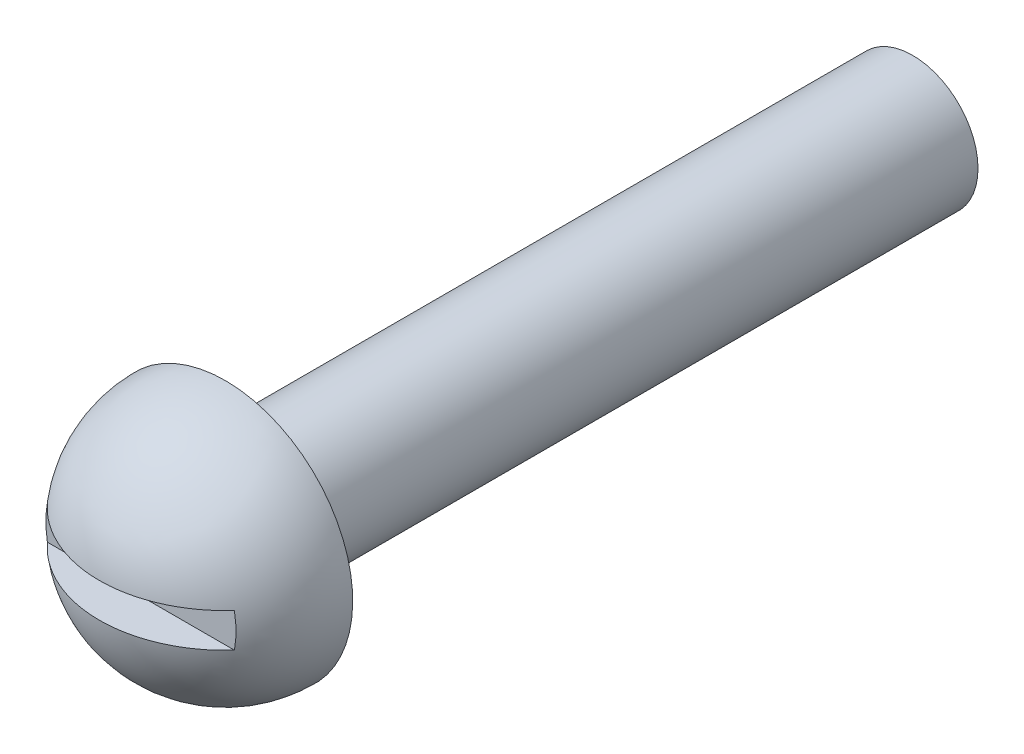
ISO-10303-21;
HEADER;
FILE_DESCRIPTION(('STEP AP214'),'2;1');
FILE_NAME('part.step','',(''),(''),'','','');
FILE_SCHEMA(('AUTOMOTIVE_DESIGN { 1 0 10303 214 1 1 1 1 }'));
ENDSEC;
DATA;
#1=APPLICATION_CONTEXT('core data for automotive mechanical design processes');
#2=APPLICATION_PROTOCOL_DEFINITION('international standard','automotive_design',2000,#1);
#3=PRODUCT_CONTEXT('',#1,'mechanical');
#4=PRODUCT('Part','Part','',(#3));
#5=PRODUCT_RELATED_PRODUCT_CATEGORY('part','',(#4));
#6=PRODUCT_DEFINITION_FORMATION('','',#4);
#7=PRODUCT_DEFINITION_CONTEXT('part definition',#1,'design');
#8=PRODUCT_DEFINITION('design','',#6,#7);
#9=PRODUCT_DEFINITION_SHAPE('','',#8);
#10=(LENGTH_UNIT() NAMED_UNIT(*) SI_UNIT(.MILLI.,.METRE.));
#11=(NAMED_UNIT(*) PLANE_ANGLE_UNIT() SI_UNIT($,.RADIAN.));
#12=(NAMED_UNIT(*) SI_UNIT($,.STERADIAN.) SOLID_ANGLE_UNIT());
#13=UNCERTAINTY_MEASURE_WITH_UNIT(LENGTH_MEASURE(1.E-05),#10,'distance_accuracy_value','');
#14=(GEOMETRIC_REPRESENTATION_CONTEXT(3) GLOBAL_UNCERTAINTY_ASSIGNED_CONTEXT((#13)) GLOBAL_UNIT_ASSIGNED_CONTEXT((#10,
#11,#12)) REPRESENTATION_CONTEXT('',''));
#15=CARTESIAN_POINT('',(0.,0.,0.));
#16=DIRECTION('',(0.,0.,1.));
#17=DIRECTION('',(1.,0.,0.));
#18=AXIS2_PLACEMENT_3D('',#15,#16,#17);
#19=CARTESIAN_POINT('',(0.,0.,25.4));
#20=DIRECTION('',(0.,0.,-1.));
#21=DIRECTION('',(-1.,0.,0.));
#22=AXIS2_PLACEMENT_3D('',#19,#20,#21);
#23=CYLINDRICAL_SURFACE('',#22,2.413);
#24=CARTESIAN_POINT('',(0.,0.,25.4));
#25=DIRECTION('',(0.,0.,1.));
#26=DIRECTION('',(1.,0.,0.));
#27=AXIS2_PLACEMENT_3D('',#24,#25,#26);
#28=CIRCLE('',#27,2.413);
#29=CARTESIAN_POINT('',(2.413,0.,25.4));
#30=VERTEX_POINT('',#29);
#31=EDGE_CURVE('E68',#30,#30,#28,.T.);
#32=ORIENTED_EDGE('',*,*,#31,.F.);
#33=EDGE_LOOP('',(#32));
#34=FACE_BOUND('',#33,.T.);
#35=CARTESIAN_POINT('',(0.,0.,0.));
#36=DIRECTION('',(0.,0.,1.));
#37=DIRECTION('',(1.,0.,0.));
#38=AXIS2_PLACEMENT_3D('',#35,#36,#37);
#39=CIRCLE('',#38,2.413);
#40=CARTESIAN_POINT('',(2.413,0.,0.));
#41=VERTEX_POINT('',#40);
#42=EDGE_CURVE('E77',#41,#41,#39,.T.);
#43=ORIENTED_EDGE('',*,*,#42,.T.);
#44=EDGE_LOOP('',(#43));
#45=FACE_BOUND('',#44,.T.);
#46=ADVANCED_FACE('F39',(#34,#45),#23,.T.);
#47=CARTESIAN_POINT('',(0.,0.,0.));
#48=DIRECTION('',(0.,0.,1.));
#49=DIRECTION('',(1.,0.,0.));
#50=AXIS2_PLACEMENT_3D('',#47,#48,#49);
#51=PLANE('',#50);
#52=ORIENTED_EDGE('',*,*,#42,.F.);
#53=EDGE_LOOP('',(#52));
#54=FACE_BOUND('',#53,.T.);
#55=ADVANCED_FACE('F98',(#54),#51,.F.);
#56=CARTESIAN_POINT('',(0.,0.,25.4));
#57=DIRECTION('',(0.,0.,-1.));
#58=DIRECTION('',(-1.,0.,0.));
#59=AXIS2_PLACEMENT_3D('',#56,#57,#58);
#60=PLANE('',#59);
#61=ORIENTED_EDGE('',*,*,#31,.T.);
#62=EDGE_LOOP('',(#61));
#63=FACE_BOUND('',#62,.T.);
#64=CARTESIAN_POINT('',(0.,0.,25.4));
#65=DIRECTION('',(0.,0.,-1.));
#66=DIRECTION('',(-1.,0.,0.));
#67=AXIS2_PLACEMENT_3D('',#64,#65,#66);
#68=CIRCLE('',#67,4.70281504894704);
#69=CARTESIAN_POINT('',(-4.70281504894704,0.,25.4));
#70=VERTEX_POINT('',#69);
#71=EDGE_CURVE('E81',#70,#70,#68,.T.);
#72=ORIENTED_EDGE('',*,*,#71,.T.);
#73=EDGE_LOOP('',(#72));
#74=FACE_BOUND('',#73,.T.);
#75=ADVANCED_FACE('F92',(#63,#74),#60,.T.);
#76=CARTESIAN_POINT('',(0.,0.,25.4));
#77=DIRECTION('',(0.,0.,-1.));
#78=DIRECTION('',(0.,1.,0.));
#79=AXIS2_PLACEMENT_3D('',#76,#77,#78);
#80=SPHERICAL_SURFACE('',#79,4.70281504894704);
#81=CARTESIAN_POINT('',(0.,0.635,25.4));
#82=DIRECTION('',(0.,1.,0.));
#83=DIRECTION('',(0.,0.,1.));
#84=AXIS2_PLACEMENT_3D('',#81,#82,#83);
#85=CIRCLE('',#84,4.65974724471218);
#86=CARTESIAN_POINT('',(3.45628281249914,0.635,28.5252765485035));
#87=VERTEX_POINT('',#86);
#88=CARTESIAN_POINT('',(-3.45628281249914,0.635,28.5252765485035));
#89=VERTEX_POINT('',#88);
#90=EDGE_CURVE('E11',#87,#89,#85,.F.);
#91=ORIENTED_EDGE('',*,*,#90,.F.);
#92=CARTESIAN_POINT('',(0.,0.,28.5252765485035));
#93=DIRECTION('',(0.,0.,-1.));
#94=DIRECTION('',(-1.,0.,0.));
#95=AXIS2_PLACEMENT_3D('',#92,#93,#94);
#96=CIRCLE('',#95,3.51413088543625);
#97=CARTESIAN_POINT('',(3.45628281249914,-0.635,28.5252765485035));
#98=VERTEX_POINT('',#97);
#99=EDGE_CURVE('E46',#98,#87,#96,.F.);
#100=ORIENTED_EDGE('',*,*,#99,.F.);
#101=CARTESIAN_POINT('',(0.,-0.635,25.4));
#102=DIRECTION('',(0.,-1.,0.));
#103=DIRECTION('',(0.,0.,-1.));
#104=AXIS2_PLACEMENT_3D('',#101,#102,#103);
#105=CIRCLE('',#104,4.65974724471218);
#106=CARTESIAN_POINT('',(-3.45628281249914,-0.635,28.5252765485035));
#107=VERTEX_POINT('',#106);
#108=EDGE_CURVE('E65',#107,#98,#105,.F.);
#109=ORIENTED_EDGE('',*,*,#108,.F.);
#110=EDGE_CURVE('E67',#89,#107,#96,.F.);
#111=ORIENTED_EDGE('',*,*,#110,.F.);
#112=EDGE_LOOP('',(#91,#100,#109,#111));
#113=FACE_BOUND('',#112,.T.);
#114=ORIENTED_EDGE('',*,*,#71,.F.);
#115=EDGE_LOOP('',(#114));
#116=FACE_BOUND('',#115,.T.);
#117=ADVANCED_FACE('F73',(#113,#116),#80,.T.);
#118=CARTESIAN_POINT('',(-4.70281504894704,0.635,31.0652765485035));
#119=DIRECTION('',(0.,1.,0.));
#120=DIRECTION('',(0.,0.,1.));
#121=AXIS2_PLACEMENT_3D('',#118,#119,#120);
#122=PLANE('',#121);
#123=ORIENTED_EDGE('',*,*,#90,.T.);
#124=DIRECTION('',(1.,0.,0.));
#125=VECTOR('',#124,1.);
#126=CARTESIAN_POINT('',(-4.70281504894704,0.635,28.5252765485035));
#127=LINE('',#126,#125);
#128=EDGE_CURVE('E75',#89,#87,#127,.T.);
#129=ORIENTED_EDGE('',*,*,#128,.T.);
#130=EDGE_LOOP('',(#123,#129));
#131=FACE_BOUND('',#130,.T.);
#132=ADVANCED_FACE('F87',(#131),#122,.F.);
#133=CARTESIAN_POINT('',(-4.70281504894704,0.635,28.5252765485035));
#134=DIRECTION('',(0.,0.,-1.));
#135=DIRECTION('',(-1.,0.,0.));
#136=AXIS2_PLACEMENT_3D('',#133,#134,#135);
#137=PLANE('',#136);
#138=ORIENTED_EDGE('',*,*,#99,.T.);
#139=ORIENTED_EDGE('',*,*,#128,.F.);
#140=ORIENTED_EDGE('',*,*,#110,.T.);
#141=DIRECTION('',(1.,0.,0.));
#142=VECTOR('',#141,1.);
#143=CARTESIAN_POINT('',(-4.70281504894704,-0.635,28.5252765485035));
#144=LINE('',#143,#142);
#145=EDGE_CURVE('E55',#107,#98,#144,.T.);
#146=ORIENTED_EDGE('',*,*,#145,.T.);
#147=EDGE_LOOP('',(#138,#139,#140,#146));
#148=FACE_BOUND('',#147,.T.);
#149=ADVANCED_FACE('F72',(#148),#137,.F.);
#150=CARTESIAN_POINT('',(-4.70281504894704,-0.635,31.0652765485035));
#151=DIRECTION('',(0.,-1.,0.));
#152=DIRECTION('',(0.,0.,-1.));
#153=AXIS2_PLACEMENT_3D('',#150,#151,#152);
#154=PLANE('',#153);
#155=ORIENTED_EDGE('',*,*,#108,.T.);
#156=ORIENTED_EDGE('',*,*,#145,.F.);
#157=EDGE_LOOP('',(#155,#156));
#158=FACE_BOUND('',#157,.T.);
#159=ADVANCED_FACE('F61',(#158),#154,.F.);
#160=CLOSED_SHELL('',(#46,#55,#75,#117,#132,#149,#159));
#161=MANIFOLD_SOLID_BREP('B2',#160);
#162=ADVANCED_BREP_SHAPE_REPRESENTATION('',(#18,#161),#14);
#163=SHAPE_DEFINITION_REPRESENTATION(#9,#162);
ENDSEC;
END-ISO-10303-21;
